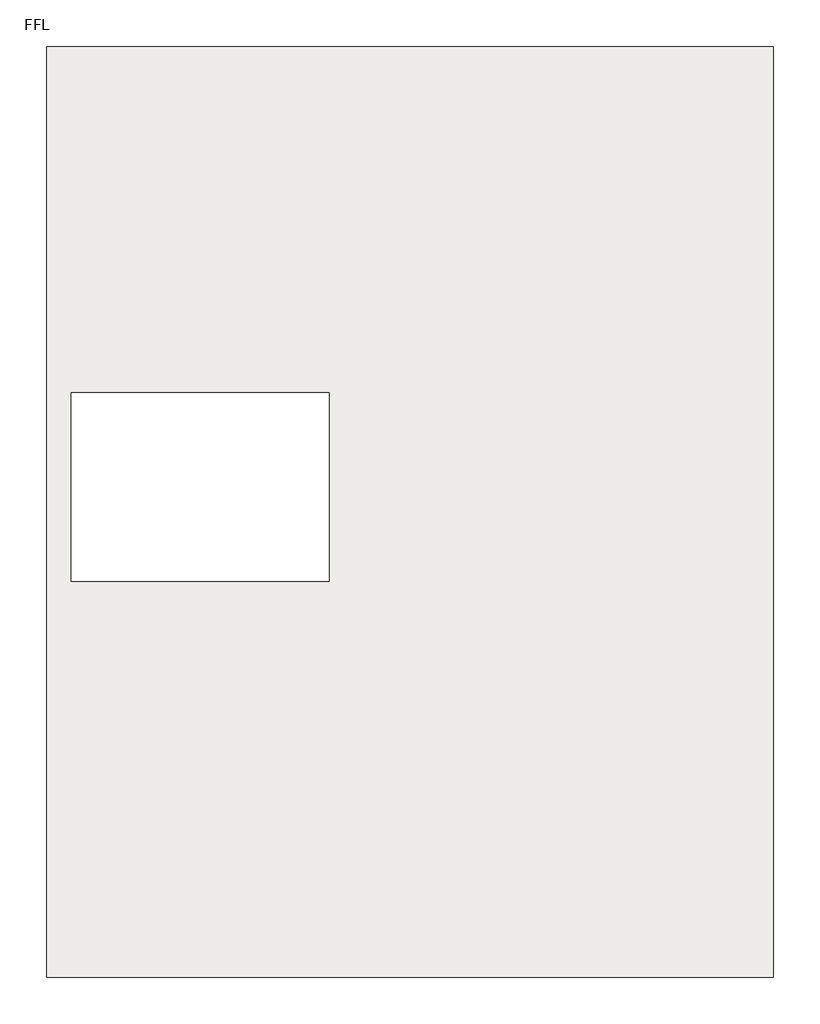
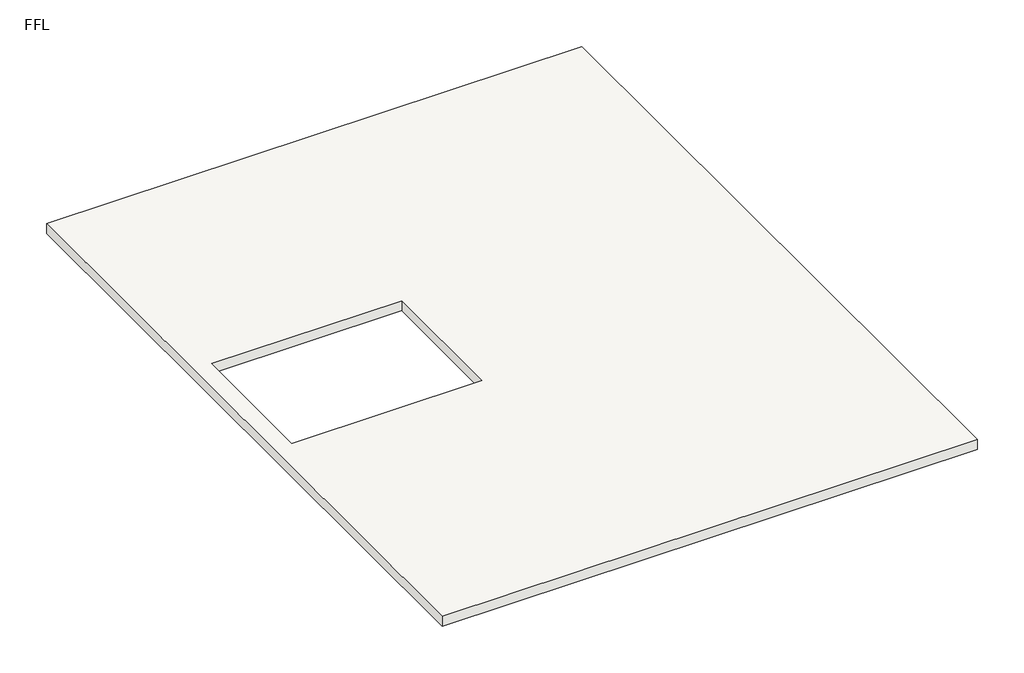
# One storey, incomplete: 1 slab.
"""IFC4 building model written with IfcOpenShell, lengths in millimetres."""

from ifc_helpers import new_model, si_unit, frame, origin, place, context, project, spatial, polyline, outline, extrude, element, save

model = new_model("IFC4")

# Units and contexts
model_context = context("Model", 3, world=origin())
ifc_project = project(units=[si_unit("LENGTHUNIT", "METRE", prefix="MILLI")], contexts=[model_context])

# Site, building, storey
site = spatial("IfcSite", under=ifc_project)
building = spatial("IfcBuilding", under=site)
storey = spatial("IfcBuildingStorey", under=building, Name="FFL", Elevation=3048.0)

# Slab
placement = place(None, origin())
element("IfcSlab", 1, ObjectType="SLAB", at=placement, inside=storey, context=model_context, shape_type="SweptSolid", body=[
    extrude(outline(polyline([(8584.6879225, 11429.2472041), (8584.6879225, 1675.6472041), (964.6879225, 1675.6472041), (964.6879225, 11429.2472041), (8584.6879225, 11429.2472041)]), holes=[polyline([(3928.8679225, 7802.1353898), (1223.7679225, 7802.1353898), (1223.7679225, 5827.2853898), (3928.8679225, 5827.2853898), (3928.8679225, 7802.1353898)])]), frame((0.0, 0.0, 3048.0), z_axis=(0.0, 0.0, 1.0), x_axis=(1.0, 0.0, 0.0)), (0.0, 0.0, 1.0), 149.9616),
])

save(model, "model.ifc")

# Revit data of these elements
# Type "SLAB"
#   Layers, outside or top first: 0.492 ft "Concrete Masonry Units _High Density" (function 1)
# Element 1 (IfcSlab, "SLAB")
#   Height Offset From Level = 0.492 ft
#   built-in parameter 1001954 = 1
#   Phase Created = New Construction
#   Materials on its faces: "Concrete Masonry Units _High Density"
# Materials
#   "Concrete Masonry Units _High Density": class "Masonry", colour RGB 181 181 181, transparency 0, Description = "Concrete masonry units", Cost = 0
